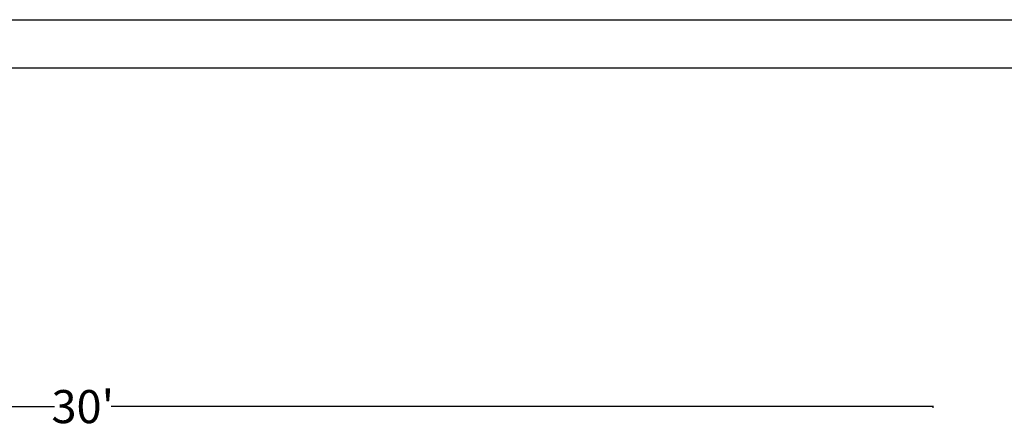
# Model space of a CAD drawing. Units: inches. Extents: x 0 to 4258, y 0 to 3769.
# Tile 29 of 30: x 3845 to 4054, y 3682 to 3769. Entities that reach past the tile are written whole.
import ezdxf

# ---------------------------------------------------------------- set-up
doc = ezdxf.new("R2010")
doc.units = ezdxf.units.IN
doc.header["$MEASUREMENT"] = 0
doc.layers.add('A-ANNO-DIMS', color=250, linetype='Continuous', lineweight=18)
doc.layers.add('A-ANNO-TTLB', color=250, linetype='Continuous', lineweight=25)
doc.styles.get("Standard").update_dxf_attribs({"font": 'arial.ttf'})
doc.dimstyles.get("Standard").update_dxf_attribs({"dimtxt": 7, "dimasz": 0.18, "dimexe": 0.18, "dimexo": 0.0625, "dimgap": 0.09, "dimtad": 0, "dimtih": 1, "dimtoh": 1, "dimzin": 0, "dimdsep": 46, "dimlunit": 3, "dimtxsty": 'Standard', "dimcen": 0.09, "dimadec": 0, "dimazin": 0, "dimtfac": 1, "dimtofl": 0, "dimtmove": 0, "dimatfit": 3, "dimfxl": 1, "dimtolj": 1, "dimtzin": 0, "dimarcsym": 0})

# ---------------------------------------------------------------- blocks, each defined once
blk = doc.blocks.new('*D24')
at = {"layer": 'A-ANNO-DIMS', "color": 0, "lineweight": -2, "transparency": 16777216}
for p, q in [((3678.8, 3686.57), (3678.8, 3687.02)), ((3678.98, 3686.84), (3852.78, 3686.84)), ((4038.62, 3686.84), (3864.83, 3686.84)), ((4038.8, 3686.57), (4038.8, 3687.02))]:
    blk.add_line(p, q, dxfattribs=at)
at = {"layer": 'A-ANNO-DIMS', "color": 0, "transparency": 16777216}
for points in [[(3678.98, 3686.87), (3678.98, 3686.81), (3678.8, 3686.84)], [(4038.62, 3686.87), (4038.62, 3686.81), (4038.8, 3686.84)]]:
    blk.add_solid(points, dxfattribs=at)
at = {"layer": 'Defpoints', "color": 0, "transparency": 16777216}
for p in [(3678.8, 3686.51), (4038.8, 3686.84), (4038.8, 3686.51)]:
    blk.add_point(p, dxfattribs=at)
at = {"layer": 'A-ANNO-DIMS', "color": 0, "transparency": 16777216, "insert": (3858.8, 3686.84), "char_height": 7, "attachment_point": 5}
blk.add_mtext("\\A1;30'", dxfattribs=at)

msp = doc.modelspace()

# ---------------------------------------------------------------- linework, layer by layer
at = {"layer": 'A-ANNO-TTLB'}
for p, q in [((3476.156, 3768.679), (4257.673, 3768.679)), ((4244.279, 3758.41), (3489.722, 3758.41))]:
    msp.add_line(p, q, dxfattribs=at)

# ---------------------------------------------------------------- dimensions: what is measured, and where the dimension line sits
at = {"layer": 'A-ANNO-DIMS'}
dim = msp.add_linear_dim(base=(4038.804, 3686.844), p1=(3678.804, 3686.506), p2=(4038.804, 3686.506), dimstyle='Standard', override={"dimclrd": 0, "dimclre": 0, "dimclrt": 0}, dxfattribs=at)
dim.commit()
dim.dimension.update_dxf_attribs({"geometry": '*D24', "text_midpoint": (3858.804, 3686.844)})

doc.saveas('drawing.dxf')
